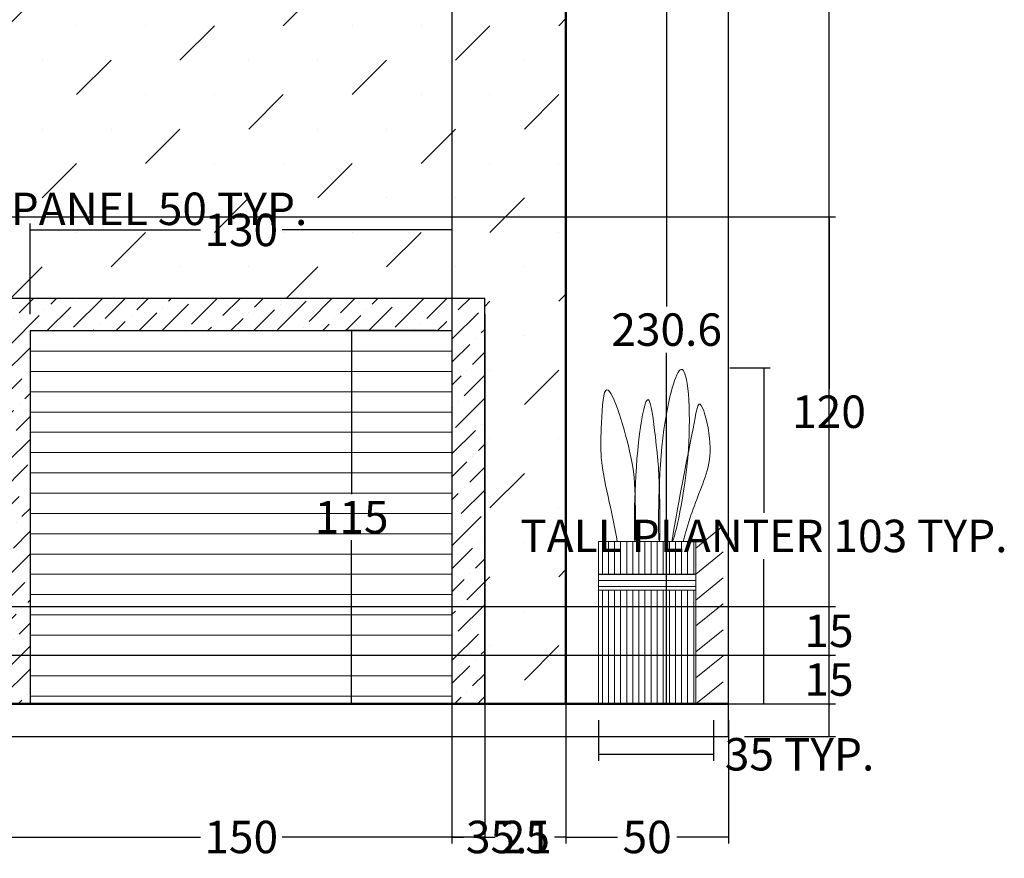
# Model space of a CAD drawing. Units: millimetres. Extents: x 301 to 1039, y -12 to 673.
# Tile 5 of 6: x 736 to 1039, y -12 to 246. Entities that reach past the tile are written whole.
import ezdxf

# ---------------------------------------------------------------- set-up
doc = ezdxf.new("R2010")
doc.units = ezdxf.units.MM
doc.header["$MEASUREMENT"] = 0
for name, color, linetype, lineweight in [('A-ANNO-DIMS', 2, 'Continuous', 18), ('A-DOOR', 4, 'Continuous', 25), ('A-DOOR-PATT', 8, 'Continuous', 13), ('A-ELEV', 8, 'Continuous', 25), ('A-WALL', 7, 'Continuous', 50), ('A-WALL-PATT', 9, 'Continuous', 13), ('L-PLNT', 3, 'Continuous', 18)]:
    doc.layers.add(name, color=color, linetype=linetype, lineweight=lineweight)
doc.styles.get("Standard").update_dxf_attribs({"font": 'arial.ttf'})
doc.dimstyles.get("Standard").update_dxf_attribs({"dimtxt": 10, "dimasz": 0.18, "dimexe": 2, "dimexo": 5, "dimgap": 2, "dimtad": 0, "dimtih": 1, "dimtoh": 1, "dimdec": 0, "dimzin": 0, "dimdsep": 46, "dimtxsty": 'Standard', "dimcen": 0.09, "dimadec": 0, "dimazin": 0, "dimtfac": 1, "dimtdec": 0, "dimtofl": 0, "dimtmove": 0, "dimatfit": 3, "dimfxl": 1, "dimtolj": 1, "dimtzin": 0, "dimarcsym": 0})

# ---------------------------------------------------------------- blocks, each defined once
blk = doc.blocks.new('*U1')
blk.add_line((0, 0), (6.81, -8.44))
blk = doc.blocks.new('*U2')
at = {"layer": 'L-PLNT', "color": 0, "linetype": 'ByBlock', "lineweight": -2, "transparency": 16777216, "rotation": 90}
for p in [(943.79, 83.09), (943.79, 75.09), (943.79, 67.09), (943.79, 59.09), (943.79, 51.09), (943.79, 43.09), (943.79, 35.09)]:
    blk.add_blockref('*U1', p, dxfattribs=at)
blk = doc.blocks.new('PLANTER-TALL')
for p, q in [((913.79, 35.09), (913.79, 85.09)), ((913.79, 85.09), (943.79, 85.09)), ((943.79, 85.09), (943.79, 35.09)), ((913.79, 75.09), (943.79, 75.09)), ((913.79, 70.09), (943.79, 70.09))]:
    blk.add_line(p, q)
for points, knots in [([(932.44, 85.09), (932.19, 88.91), (932, 117.56), (940.64, 148.58), (943.41, 110.75), (932.62, 67.84), (940.69, 108.37), (944.93, 130.41), (949.97, 112.97), (945.67, 102.5), (941.16, 90.48), (939.89, 85.09)], [190.612749, 190.612749, 190.612749, 190.612749, 217.894774, 237.177461, 261.995493, 290.738764, 329.494028, 333.833671, 341.635675, 361.055373, 377.63197, 377.63197, 377.63197, 377.63197]), ([(919.6, 85.09), (918.81, 89.12), (917.13, 97.69), (914.28, 109.64), (914.65, 119.96), (915.42, 140.89), (924.57, 111.13), (925.2, 100.17), (925.2, 87.12), (925.13, 85.09)], [0, 0, 0, 0, 12.444322, 26.420596, 35.223716, 47.132736, 67.219262, 83.208341, 95.201321, 95.201321, 95.201321, 95.201321]), ([(924.96, 85.09), (924.77, 89.03), (924.72, 111.77), (929.35, 134.6), (931.92, 112.35), (932.77, 102.84), (932.74, 87.27), (932.64, 85.09)], [102.717678, 102.717678, 102.717678, 102.717678, 128.408935, 139.329582, 151.017137, 169.163832, 183.363914, 183.363914, 183.363914, 183.363914])]:
    blk.add_open_spline(points, degree=3, knots=knots)
blk = doc.blocks.new('*D10')
at = {"layer": 'A-ANNO-DIMS', "color": 0, "lineweight": -2, "transparency": 16777216}
for p, q in [((633.79, 185.09), (633.79, 189.59)), ((683.79, 185.09), (683.79, 189.59)), ((633.97, 187.59), (683.61, 187.59)), ((683.79, 187.59), (683.97, 187.59))]:
    blk.add_line(p, q, dxfattribs=at)
at = {"layer": 'A-ANNO-DIMS', "color": 0, "transparency": 16777216}
for points in [[(633.97, 187.62), (633.97, 187.56), (633.79, 187.59)], [(683.61, 187.62), (683.61, 187.56), (683.79, 187.59)]]:
    blk.add_solid(points, dxfattribs=at)
at = {"layer": 'Defpoints', "color": 0, "transparency": 16777216}
for p in [(683.79, 187.59), (633.79, 180.09), (683.79, 180.09)]:
    blk.add_point(p, dxfattribs=at)
at = {"layer": 'A-ANNO-DIMS', "color": 0, "transparency": 16777216, "insert": (757.8, 187.59), "char_height": 10, "attachment_point": 5}
blk.add_mtext('\\A1;DOOR PANEL 50 TYP.', dxfattribs=at)
blk = doc.blocks.new('*D18')
at = {"layer": 'A-ANNO-DIMS', "color": 0, "lineweight": -2, "transparency": 16777216}
for p, q in [((954.2, 138.57), (966.72, 138.57)), ((964.72, 138.39), (964.72, 93.94)), ((964.72, 35.27), (964.72, 79.72)), ((954.2, 35.09), (966.72, 35.09))]:
    blk.add_line(p, q, dxfattribs=at)
at = {"layer": 'A-ANNO-DIMS', "color": 0, "transparency": 16777216}
for points in [[(964.69, 138.39), (964.75, 138.39), (964.72, 138.57)], [(964.69, 35.27), (964.75, 35.27), (964.72, 35.09)]]:
    blk.add_solid(points, dxfattribs=at)
at = {"layer": 'Defpoints', "color": 0, "transparency": 16777216}
for p in [(949.2, 138.57), (964.72, 138.57), (949.2, 35.09)]:
    blk.add_point(p, dxfattribs=at)
at = {"layer": 'A-ANNO-DIMS', "color": 0, "transparency": 16777216, "insert": (964.72, 86.83), "char_height": 10, "attachment_point": 5}
blk.add_mtext('\\A1;TALL PLANTER 103 TYP.', dxfattribs=at)
blk = doc.blocks.new('*D19')
at = {"layer": 'A-ANNO-DIMS', "color": 0, "lineweight": -2, "transparency": 16777216}
for p, q in [((913.79, 30.09), (913.79, 17.57)), ((949.2, 30.09), (949.2, 17.57)), ((913.97, 19.57), (949.02, 19.57)), ((949.2, 19.57), (949.38, 19.57))]:
    blk.add_line(p, q, dxfattribs=at)
at = {"layer": 'A-ANNO-DIMS', "color": 0, "transparency": 16777216}
for points in [[(913.97, 19.6), (913.97, 19.54), (913.79, 19.57)], [(949.02, 19.6), (949.02, 19.54), (949.2, 19.57)]]:
    blk.add_solid(points, dxfattribs=at)
at = {"layer": 'Defpoints', "color": 0, "transparency": 16777216}
for p in [(913.79, 35.09), (949.2, 35.09), (949.2, 19.57)]:
    blk.add_point(p, dxfattribs=at)
at = {"layer": 'A-ANNO-DIMS', "color": 0, "transparency": 16777216, "insert": (975.72, 19.57), "char_height": 10, "attachment_point": 5}
blk.add_mtext('\\A1;35 TYP.', dxfattribs=at)
blk = doc.blocks.new('*D20')
at = {"layer": 'A-ANNO-DIMS', "color": 0, "lineweight": -2, "transparency": 16777216}
for p, q in [((343.79, 30.09), (343.79, 668.09)), ((953.79, 30.09), (953.79, 668.09)), ((343.97, 666.09), (635.73, 666.09)), ((953.61, 666.09), (661.85, 666.09))]:
    blk.add_line(p, q, dxfattribs=at)
at = {"layer": 'A-ANNO-DIMS', "color": 0, "transparency": 16777216}
for points in [[(343.97, 666.12), (343.97, 666.06), (343.79, 666.09)], [(953.61, 666.12), (953.61, 666.06), (953.79, 666.09)]]:
    blk.add_solid(points, dxfattribs=at)
at = {"layer": 'Defpoints', "color": 0, "transparency": 16777216}
for p in [(953.79, 666.09), (343.79, 25.09), (953.79, 25.09)]:
    blk.add_point(p, dxfattribs=at)
at = {"layer": 'A-ANNO-DIMS', "color": 0, "transparency": 16777216, "insert": (648.79, 666.09), "char_height": 10, "attachment_point": 5}
blk.add_mtext('\\A1;610', dxfattribs=at)
blk = doc.blocks.new('*D21')
at = {"layer": 'A-ANNO-DIMS', "color": 0, "lineweight": -2, "transparency": 16777216}
for p, q in [((905.87, 635.09), (986.79, 635.09)), ((984.79, 634.91), (984.79, 337.19)), ((984.79, 25.27), (984.79, 322.98)), ((958.79, 25.09), (986.79, 25.09))]:
    blk.add_line(p, q, dxfattribs=at)
at = {"layer": 'A-ANNO-DIMS', "color": 0, "transparency": 16777216}
for points in [[(984.76, 634.91), (984.82, 634.91), (984.79, 635.09)], [(984.76, 25.27), (984.82, 25.27), (984.79, 25.09)]]:
    blk.add_solid(points, dxfattribs=at)
at = {"layer": 'Defpoints', "color": 0, "transparency": 16777216}
for p in [(900.87, 635.09), (984.79, 635.09), (953.79, 25.09)]:
    blk.add_point(p, dxfattribs=at)
at = {"layer": 'A-ANNO-DIMS', "color": 0, "transparency": 16777216, "insert": (984.79, 330.09), "char_height": 10, "attachment_point": 5}
blk.add_mtext('\\A1;610', dxfattribs=at)
blk = doc.blocks.new('*D28')
at = {"layer": 'A-ANNO-DIMS', "color": 0, "lineweight": -2, "transparency": 16777216}
for p, q in [((728.79, 155.09), (728.79, -7.91)), ((878.79, 155.09), (878.79, -7.91)), ((728.97, -5.91), (791.23, -5.91)), ((878.61, -5.91), (816.35, -5.91))]:
    blk.add_line(p, q, dxfattribs=at)
at = {"layer": 'A-ANNO-DIMS', "color": 0, "transparency": 16777216}
for points in [[(728.97, -5.88), (728.97, -5.94), (728.79, -5.91)], [(878.61, -5.88), (878.61, -5.94), (878.79, -5.91)]]:
    blk.add_solid(points, dxfattribs=at)
at = {"layer": 'Defpoints', "color": 0, "transparency": 16777216}
for p in [(728.79, 160.09), (878.79, 160.09), (878.79, -5.91)]:
    blk.add_point(p, dxfattribs=at)
at = {"layer": 'A-ANNO-DIMS', "color": 0, "transparency": 16777216, "insert": (803.79, -5.91), "char_height": 10, "attachment_point": 5}
blk.add_mtext('\\A1;150', dxfattribs=at)
blk = doc.blocks.new('*D29')
at = {"layer": 'A-ANNO-DIMS', "color": 0, "lineweight": -2, "transparency": 16777216}
for p, q in [((878.79, 30.09), (878.79, -7.91)), ((903.79, 30.09), (903.79, -7.91)), ((878.97, -5.91), (882, -5.91)), ((903.61, -5.91), (900.57, -5.91))]:
    blk.add_line(p, q, dxfattribs=at)
at = {"layer": 'A-ANNO-DIMS', "color": 0, "transparency": 16777216}
for points in [[(878.97, -5.88), (878.97, -5.94), (878.79, -5.91)], [(903.61, -5.88), (903.61, -5.94), (903.79, -5.91)]]:
    blk.add_solid(points, dxfattribs=at)
at = {"layer": 'Defpoints', "color": 0, "transparency": 16777216}
for p in [(878.79, 35.09), (903.79, 35.09), (903.79, -5.91)]:
    blk.add_point(p, dxfattribs=at)
at = {"layer": 'A-ANNO-DIMS', "color": 0, "transparency": 16777216, "insert": (891.29, -5.91), "char_height": 10, "attachment_point": 5}
blk.add_mtext('\\A1;25', dxfattribs=at)
blk = doc.blocks.new('*D30')
at = {"layer": 'A-ANNO-DIMS', "color": 0, "lineweight": -2, "transparency": 16777216}
for p, q in [((903.79, 30.09), (903.79, -7.91)), ((953.79, 30.09), (953.79, -7.91)), ((903.97, -5.91), (919.64, -5.91)), ((953.61, -5.91), (937.93, -5.91))]:
    blk.add_line(p, q, dxfattribs=at)
at = {"layer": 'A-ANNO-DIMS', "color": 0, "transparency": 16777216}
for points in [[(903.97, -5.88), (903.97, -5.94), (903.79, -5.91)], [(953.61, -5.88), (953.61, -5.94), (953.79, -5.91)]]:
    blk.add_solid(points, dxfattribs=at)
at = {"layer": 'Defpoints', "color": 0, "transparency": 16777216}
for p in [(903.79, 35.09), (953.79, 35.09), (953.79, -5.91)]:
    blk.add_point(p, dxfattribs=at)
at = {"layer": 'A-ANNO-DIMS', "color": 0, "transparency": 16777216, "insert": (928.79, -5.91), "char_height": 10, "attachment_point": 5}
blk.add_mtext('\\A1;50', dxfattribs=at)
blk = doc.blocks.new('*D38')
at = {"layer": 'A-ANNO-DIMS', "color": 0, "lineweight": -2, "transparency": 16777216}
for p, q in [((908.79, 265.67), (936.79, 265.67)), ((934.79, 265.49), (934.79, 157.49)), ((934.79, 35.27), (934.79, 143.27)), ((908.79, 35.09), (936.79, 35.09))]:
    blk.add_line(p, q, dxfattribs=at)
at = {"layer": 'A-ANNO-DIMS', "color": 0, "transparency": 16777216}
for points in [[(934.76, 265.49), (934.82, 265.49), (934.79, 265.67)], [(934.76, 35.27), (934.82, 35.27), (934.79, 35.09)]]:
    blk.add_solid(points, dxfattribs=at)
at = {"layer": 'Defpoints', "color": 0, "transparency": 16777216}
for p in [(903.79, 265.67), (903.79, 35.09), (934.79, 35.09)]:
    blk.add_point(p, dxfattribs=at)
at = {"layer": 'A-ANNO-DIMS', "color": 0, "transparency": 16777216, "insert": (934.79, 150.38), "char_height": 10, "attachment_point": 5}
blk.add_mtext('\\A1;230.6', dxfattribs=at)
blk = doc.blocks.new('*D41')
at = {"layer": 'A-ANNO-DIMS', "color": 0, "lineweight": -2, "transparency": 16777216}
for p, q in [((863.79, 150.09), (835.79, 150.09)), ((837.79, 149.91), (837.79, 99.69)), ((837.79, 35.27), (837.79, 85.48)), ((863.79, 35.09), (835.79, 35.09))]:
    blk.add_line(p, q, dxfattribs=at)
at = {"layer": 'A-ANNO-DIMS', "color": 0, "transparency": 16777216}
for points in [[(837.76, 149.91), (837.82, 149.91), (837.79, 150.09)], [(837.76, 35.27), (837.82, 35.27), (837.79, 35.09)]]:
    blk.add_solid(points, dxfattribs=at)
at = {"layer": 'Defpoints', "color": 0, "transparency": 16777216}
for p in [(837.79, 150.09), (868.79, 150.09), (868.79, 35.09)]:
    blk.add_point(p, dxfattribs=at)
at = {"layer": 'A-ANNO-DIMS', "color": 0, "transparency": 16777216, "insert": (837.79, 92.59), "char_height": 10, "attachment_point": 5}
blk.add_mtext('\\A1;115', dxfattribs=at)
blk = doc.blocks.new('*D42')
at = {"layer": 'A-ANNO-DIMS', "color": 0, "lineweight": -2, "transparency": 16777216}
for p, q in [((738.79, 155.09), (738.79, 183.09)), ((868.79, 155.09), (868.79, 183.09)), ((738.97, 181.09), (791.23, 181.09)), ((868.61, 181.09), (816.35, 181.09))]:
    blk.add_line(p, q, dxfattribs=at)
at = {"layer": 'A-ANNO-DIMS', "color": 0, "transparency": 16777216}
for points in [[(738.97, 181.12), (738.97, 181.06), (738.79, 181.09)], [(868.61, 181.12), (868.61, 181.06), (868.79, 181.09)]]:
    blk.add_solid(points, dxfattribs=at)
at = {"layer": 'Defpoints', "color": 0, "transparency": 16777216}
for p in [(868.79, 181.09), (738.79, 150.09), (868.79, 150.09)]:
    blk.add_point(p, dxfattribs=at)
at = {"layer": 'A-ANNO-DIMS', "color": 0, "transparency": 16777216, "insert": (803.79, 181.09), "char_height": 10, "attachment_point": 5}
blk.add_mtext('\\A1;130', dxfattribs=at)
blk = doc.blocks.new('*D69')
at = {"layer": 'A-ANNO-DIMS', "color": 0, "lineweight": -2, "transparency": 16777216}
for p, q in [((708.788413, 50.088152), (986.788413, 50.088152)), ((984.788413, 50.268152), (984.788413, 50.448152)), ((708.788413, 35.088152), (986.788413, 35.088152)), ((984.788413, 34.908152), (984.788413, 34.728152))]:
    blk.add_line(p, q, dxfattribs=at)
at = {"layer": 'A-ANNO-DIMS', "color": 0, "transparency": 16777216}
for points in [[(984.758413, 50.268152), (984.818413, 50.268152), (984.788413, 50.088152)], [(984.758413, 34.908152), (984.818413, 34.908152), (984.788413, 35.088152)]]:
    blk.add_solid(points, dxfattribs=at)
at = {"layer": 'Defpoints', "color": 0, "transparency": 16777216}
for p in [(703.788413, 50.088152), (984.788413, 50.088152), (703.788413, 35.088152)]:
    blk.add_point(p, dxfattribs=at)
at = {"layer": 'A-ANNO-DIMS', "color": 0, "transparency": 16777216, "insert": (984.788413, 42.588152), "char_height": 10, "attachment_point": 5}
blk.add_mtext('\\A1;15', dxfattribs=at)
blk = doc.blocks.new('*D70')
at = {"layer": 'A-ANNO-DIMS', "color": 0, "lineweight": -2, "transparency": 16777216}
for p, q in [((708.788413, 65.088152), (986.788413, 65.088152)), ((984.788413, 65.268152), (984.788413, 65.448152)), ((708.788413, 50.088152), (986.788413, 50.088152)), ((984.788413, 49.908152), (984.788413, 49.728152))]:
    blk.add_line(p, q, dxfattribs=at)
at = {"layer": 'A-ANNO-DIMS', "color": 0, "transparency": 16777216}
for points in [[(984.758413, 65.268152), (984.818413, 65.268152), (984.788413, 65.088152)], [(984.758413, 49.908152), (984.818413, 49.908152), (984.788413, 50.088152)]]:
    blk.add_solid(points, dxfattribs=at)
at = {"layer": 'Defpoints', "color": 0, "transparency": 16777216}
for p in [(703.788413, 65.088152), (984.788413, 65.088152), (703.788413, 50.088152)]:
    blk.add_point(p, dxfattribs=at)
at = {"layer": 'A-ANNO-DIMS', "color": 0, "transparency": 16777216, "insert": (984.788413, 57.588152), "char_height": 10, "attachment_point": 5}
blk.add_mtext('\\A1;15', dxfattribs=at)
blk = doc.blocks.new('*D71')
at = {"layer": 'A-ANNO-DIMS', "color": 0, "lineweight": -2, "transparency": 16777216}
for p, q in [((693.79, 185.09), (986.79, 185.09)), ((984.79, 184.91), (984.79, 132.19)), ((984.79, 65.27), (984.79, 117.98)), ((693.79, 65.09), (986.79, 65.09))]:
    blk.add_line(p, q, dxfattribs=at)
at = {"layer": 'A-ANNO-DIMS', "color": 0, "transparency": 16777216}
for points in [[(984.76, 184.91), (984.82, 184.91), (984.79, 185.09)], [(984.76, 65.27), (984.82, 65.27), (984.79, 65.09)]]:
    blk.add_solid(points, dxfattribs=at)
at = {"layer": 'Defpoints', "color": 0, "transparency": 16777216}
for p in [(688.79, 185.09), (984.79, 185.09), (688.79, 65.09)]:
    blk.add_point(p, dxfattribs=at)
at = {"layer": 'A-ANNO-DIMS', "color": 0, "transparency": 16777216, "insert": (984.79, 125.09), "char_height": 10, "attachment_point": 5}
blk.add_mtext('\\A1;120', dxfattribs=at)
blk = doc.blocks.new('*D75')
at = {"layer": 'A-ANNO-DIMS', "color": 0, "lineweight": -2, "transparency": 16777216}
for p, q in [((868.69, 285.26), (868.69, -7.91)), ((903.79, 260.67), (903.79, -7.91)), ((868.87, -5.91), (872.22, -5.91)), ((903.61, -5.91), (900.26, -5.91))]:
    blk.add_line(p, q, dxfattribs=at)
at = {"layer": 'A-ANNO-DIMS', "color": 0, "transparency": 16777216}
for points in [[(868.87, -5.88), (868.87, -5.94), (868.69, -5.91)], [(903.61, -5.88), (903.61, -5.94), (903.79, -5.91)]]:
    blk.add_solid(points, dxfattribs=at)
at = {"layer": 'Defpoints', "color": 0, "transparency": 16777216}
for p in [(868.69, 290.26), (903.79, 265.67), (903.79, -5.91)]:
    blk.add_point(p, dxfattribs=at)
at = {"layer": 'A-ANNO-DIMS', "color": 0, "transparency": 16777216, "insert": (886.24, -5.91), "char_height": 10, "attachment_point": 5}
blk.add_mtext('\\A1;35.1', dxfattribs=at)

msp = doc.modelspace()

# ---------------------------------------------------------------- hatches: boundary and pattern name
at = {"layer": 'A-DOOR-PATT'}
h = msp.add_hatch(dxfattribs=at)
h.set_pattern_fill('ANSI31', color=256, scale=50, angle=135)
h.paths.add_polyline_path([(868.788, 150.088), (738.788, 150.088), (738.788, 35.088), (868.788, 35.088)])
at = {"layer": 'A-WALL-PATT'}
h = msp.add_hatch(dxfattribs=at)
h.set_pattern_fill('MUDST', color=256, scale=60, angle=45)
edge = h.paths.add_edge_path()
edge.add_line((703.788, 505.088), (403.788, 505.088))
edge.add_line((403.788, 505.088), (403.788, 335.088))
edge.add_line((403.788, 335.088), (448.788, 335.088))
edge.add_line((448.788, 335.088), (448.788, 400.52))
edge.add_line((448.788, 400.52), (448.788, 440.088))
edge.add_line((448.788, 440.088), (633.788, 440.088))
edge.add_line((633.788, 440.088), (633.788, 400.52))
edge.add_line((633.788, 400.52), (633.788, 335.088))
edge.add_line((633.788, 335.088), (673.88, 335.088))
edge.add_spline(control_points=[(673.88, 335.088), (673.929, 335.734), (674.283, 339.462), (675.587, 346.794), (678.602, 339.909), (679.226, 336.718), (679.369, 335.088)], knot_values=[26.7052686, 26.7052686, 26.7052686, 26.7052686, 28.3156814, 35.5227919, 39.6456178, 44.5318346, 44.5318346, 44.5318346, 44.5318346], degree=3, periodic=0)
edge.add_line((679.369, 335.088), (703.788, 335.088))
edge.add_line((703.788, 335.088), (703.788, 505.088))
h.paths.add_polyline_path([(681.292, 397.334, -1), (651.292, 397.334, -1)], flags=16)
h.paths.add_polyline_path([(679.292, 397.334, -1), (653.292, 397.334, -1)], flags=0)
h.paths.add_polyline_path([(448.788, 333.088), (403.788, 333.088), (403.788, 285.088), (448.788, 285.088)])
h.paths.add_polyline_path([(613.788, 260.088), (713.788, 260.088), (713.788, 285.088), (403.788, 285.088), (393.788, 285.088), (393.788, 35.088), (403.788, 35.088), (613.788, 35.088)])
h.paths.add_polyline_path([(578.788, 215.088), (578.788, 105.088), (428.788, 105.088), (428.788, 215.088)], flags=16)
h.paths.add_polyline_path([(501.288, 210.088), (501.288, 185.088), (433.788, 185.088), (433.788, 210.088)], flags=0)
h.paths.add_polyline_path([(501.288, 180.088), (501.288, 110.088), (433.788, 110.088), (433.788, 180.088)], flags=0)
h.paths.add_polyline_path([(506.288, 210.088), (573.788, 210.088), (573.788, 185.088), (506.288, 185.088)], flags=0)
h.paths.add_polyline_path([(506.288, 180.088), (573.788, 180.088), (573.788, 110.088), (506.288, 110.088)], flags=0)
edge = h.paths.add_edge_path()
edge.add_spline(control_points=[(675.148, 309.006), (675.282, 309.92), (671.965, 311.304), (670.019, 313.17), (668.379, 316.485), (667.076, 320.028), (669.149, 324.142), (672.687, 322.877), (673.644, 321.553), (673.786, 321.296)], knot_values=[12.4980994, 12.4980994, 12.4980994, 12.4980994, 15.7345293, 18.1242776, 22.0598536, 26.1694355, 29.2709867, 33.3603853, 34.273637, 34.273637, 34.273637, 34.273637], degree=3, periodic=0)
edge.add_spline(control_points=[(673.786, 321.296), (673.373, 322.666), (672.565, 324.662), (673.805, 325.84), (674.246, 326.099)], knot_values=[12.3304253, 12.3304253, 12.3304253, 12.3304253, 16.1943692, 17.6683934, 17.6683934, 17.6683934, 17.6683934], degree=3, periodic=0)
edge.add_spline(control_points=[(674.246, 326.099), (673.92, 328.298), (673.697, 330.39), (673.774, 333.088)], knot_values=[46.2924512, 46.2924512, 46.2924512, 46.2924512, 53.8278009, 53.8278009, 53.8278009, 53.8278009], degree=3, periodic=0)
edge.add_line((673.774, 333.088), (648.788, 333.088))
edge.add_line((648.788, 333.088), (648.788, 285.088))
edge.add_line((648.788, 285.088), (666.788, 285.088))
edge.add_line((666.788, 285.088), (664.215, 309.96))
edge.add_arc((676.288, 385.148), 76.15, 260.87778, 269.14183)
edge = h.paths.add_edge_path()
edge.add_line((703.788, 333.088), (679.453, 333.088))
edge.add_spline(control_points=[(679.453, 333.088), (679.452, 331.277), (679.21, 329.205), (678.936, 327.067), (678.889, 326.706)], knot_values=[17.8386285, 17.8386285, 17.8386285, 17.8386285, 23.5111371, 24.6594022, 24.6594022, 24.6594022, 24.6594022], degree=3, periodic=0)
edge.add_spline(control_points=[(678.889, 326.706), (678.729, 326.741), (678.565, 326.771), (678.396, 326.794)], knot_values=[21.2892091, 21.2892091, 21.2892091, 21.2892091, 21.7264211, 21.7264211, 21.7264211, 21.7264211], degree=3, periodic=0)
edge.add_spline(control_points=[(678.396, 326.794), (678.233, 326.816), (678.067, 326.832), (677.898, 326.842)], knot_values=[20.8675669, 20.8675669, 20.8675669, 20.8675669, 21.2892091, 21.2892091, 21.2892091, 21.2892091], degree=3, periodic=0)
edge.add_spline(control_points=[(677.898, 326.842), (676.995, 326.898), (676.024, 326.786), (675.195, 326.517)], knot_values=[18.611077, 18.611077, 18.611077, 18.611077, 20.8675669, 20.8675669, 20.8675669, 20.8675669], degree=3, periodic=0)
edge.add_spline(control_points=[(675.195, 326.517), (675.029, 326.464), (674.869, 326.404), (674.716, 326.337)], knot_values=[18.1593829, 18.1593829, 18.1593829, 18.1593829, 18.611077, 18.611077, 18.611077, 18.611077], degree=3, periodic=0)
edge.add_spline(control_points=[(674.716, 326.337), (674.55, 326.265), (674.392, 326.186), (674.246, 326.099)], knot_values=[17.6683934, 17.6683934, 17.6683934, 17.6683934, 18.1593829, 18.1593829, 18.1593829, 18.1593829], degree=3, periodic=0)
edge.add_spline(control_points=[(674.246, 326.099), (673.805, 325.84), (672.565, 324.662), (673.373, 322.666), (673.786, 321.296)], knot_values=[12.3304253, 12.3304253, 12.3304253, 12.3304253, 13.8044495, 17.6683934, 17.6683934, 17.6683934, 17.6683934], degree=3, periodic=0)
edge.add_spline(control_points=[(673.786, 321.296), (674.162, 320.613), (674.301, 319.823), (674.341, 318.987)], knot_values=[10.0649388, 10.0649388, 10.0649388, 10.0649388, 12.4980994, 12.4980994, 12.4980994, 12.4980994], degree=3, periodic=0)
edge.add_spline(control_points=[(674.341, 318.987), (674.206, 319.737), (674.024, 320.504), (673.786, 321.296)], knot_values=[10.094462, 10.094462, 10.094462, 10.094462, 12.3304253, 12.3304253, 12.3304253, 12.3304253], degree=3, periodic=0)
edge.add_spline(control_points=[(673.786, 321.296), (673.644, 321.553), (672.687, 322.877), (669.149, 324.142), (667.076, 320.028), (668.379, 316.485), (670.019, 313.17), (671.965, 311.304), (675.282, 309.92), (675.148, 309.006)], knot_values=[12.4980994, 12.4980994, 12.4980994, 12.4980994, 13.4113511, 17.5007497, 20.6023009, 24.7118828, 28.6474588, 31.0372071, 34.273637, 34.273637, 34.273637, 34.273637], degree=3, periodic=0)
edge.add_arc((676.288, 385.148), 76.15, 260.87778, 269.14183, ccw=False)
edge.add_line((664.215, 309.96), (666.788, 285.088))
edge.add_line((666.788, 285.088), (703.788, 285.088))
edge.add_line((703.788, 285.088), (703.788, 333.088))
h.paths.add_polyline_path([(687.234, 308.777), (684.887, 286.088), (667.69, 286.088), (665.343, 308.777, 0.0712952)], flags=16)
h.paths.add_polyline_path([(903.788, 265.672), (713.788, 265.672), (713.788, 260.088), (703.788, 260.088), (703.788, 35.088), (728.788, 35.088), (728.788, 160.088), (878.788, 160.088), (878.788, 35.088), (903.788, 35.088)])
h = msp.add_hatch(dxfattribs=at)
h.set_pattern_fill('ANSI36', color=256, scale=40)
h.paths.add_polyline_path([(878.788, 160.088), (728.788, 160.088), (728.788, 35.088), (738.788, 35.088), (738.788, 150.088), (868.788, 150.088), (868.788, 35.088), (878.788, 35.088)])
at = {"layer": 'L-PLNT'}
h = msp.add_hatch(dxfattribs=at)
h.set_pattern_fill('ANSI31', color=256, scale=15, angle=45)
edge = h.paths.add_edge_path()
edge.add_line((943.788, 85.088), (936.592, 85.088))
edge.add_spline(control_points=[(936.592, 85.088), (936.558, 85.041), (936.535, 85.042), (936.521, 85.088)], knot_values=[290.7387637, 290.7387637, 290.7387637, 290.7387637, 292.5163462, 292.5163462, 292.5163462, 292.5163462], degree=3, periodic=0)
edge.add_line((936.521, 85.088), (913.788, 85.088))
edge.add_line((913.788, 85.088), (913.788, 75.088))
edge.add_line((913.788, 75.088), (943.788, 75.088))
edge.add_line((943.788, 75.088), (943.788, 85.088))
h.paths.add_polyline_path([(943.788, 70.088), (913.788, 70.088), (913.788, 35.088), (943.788, 35.088)])
h = msp.add_hatch(dxfattribs=at)
h.set_pattern_fill('ANSI31', color=256, scale=15, angle=135)
h.paths.add_polyline_path([(943.788, 75.088), (913.788, 75.088), (913.788, 70.088), (943.788, 70.088)])

# ---------------------------------------------------------------- linework, layer by layer
at = {"layer": 'A-DOOR'}
for p, q in [((728.788, 160.088), (878.788, 160.088)), ((878.788, 35.088), (878.788, 160.088)), ((738.788, 150.088), (868.788, 150.088)), ((738.788, 150.088), (738.788, 35.088)), ((868.788, 35.088), (868.788, 150.088))]:
    msp.add_line(p, q, dxfattribs=at)
at = {"layer": 'A-ELEV'}
for p, q in [((953.788, 25.088), (953.788, 35.088)), ((618.788, 25.088), (953.788, 25.088))]:
    msp.add_line(p, q, dxfattribs=at)
at = {"layer": 'A-WALL'}
for p, q in [((903.788, 35.088), (903.788, 585.088)), ((953.788, 35.088), (403.788, 35.088)), ((953.788, 35.088), (903.788, 35.088))]:
    msp.add_line(p, q, dxfattribs=at)

# ---------------------------------------------------------------- block references
at = {"layer": 'L-PLNT'}
for name in ['PLANTER-TALL', '*U2']:
    msp.add_blockref(name, (0, 0), dxfattribs=at)

# ---------------------------------------------------------------- dimensions: what is measured, and where the dimension line sits
at = {"layer": 'A-ANNO-DIMS'}
for base, p1, p2, override, picture, middle in [((953.788, 666.088), (343.788, 25.088), (953.788, 25.088), {"dimdec": 0, "dimlfac": 1, "dimrnd": 0, "dimzin": 0, "dimdsep": 46, "dimlunit": 2}, '*D20', (648.788, 666.088)), ((903.788, -5.912), (868.687, 290.264), (903.788, 265.672), {"dimdec": 1, "dimlfac": 1, "dimrnd": 0, "dimzin": 0, "dimdsep": 46, "dimlunit": 2}, '*D75', (886.238, -5.912)), ((868.788, 181.088), (738.788, 150.088), (868.788, 150.088), {"dimdec": 0, "dimlfac": 1, "dimrnd": 0, "dimzin": 0, "dimdsep": 46, "dimlunit": 2}, '*D42', (803.788, 181.088)), ((878.788, -5.912), (728.788, 160.088), (878.788, 160.088), {"dimdec": 0, "dimlfac": 1, "dimrnd": 0, "dimzin": 0, "dimdsep": 46, "dimlunit": 2}, '*D28', (803.788, -5.912)), ((903.788, -5.912), (878.788, 35.088), (903.788, 35.088), {"dimdec": 0, "dimlfac": 1, "dimrnd": 0, "dimzin": 0, "dimdsep": 46, "dimlunit": 2}, '*D29', (891.288, -5.912)), ((953.788, -5.912), (903.788, 35.088), (953.788, 35.088), {"dimdec": 0, "dimlfac": 1, "dimrnd": 0, "dimzin": 0, "dimdsep": 46, "dimlunit": 2}, '*D30', (928.788, -5.912))]:
    dim = msp.add_linear_dim(base=base, p1=p1, p2=p2, dimstyle='Standard', override=override, dxfattribs=at)
    dim.commit()
    dim.dimension.update_dxf_attribs({"geometry": picture, "text_midpoint": middle})
for base, p1, p2, angle, override, picture, middle in [((984.788, 635.088), (953.788, 25.088), (900.87, 635.088), 90, {"dimdec": 0, "dimlfac": 1, "dimrnd": 0, "dimzin": 0, "dimdsep": 46, "dimlunit": 2}, '*D21', (984.788, 330.088)), ((934.788, 35.088), (903.788, 265.672), (903.788, 35.088), 270, {"dimdec": 1, "dimlfac": 1, "dimrnd": 0, "dimzin": 0, "dimdsep": 46, "dimlunit": 2}, '*D38', (934.788, 150.38)), ((984.788, 185.088), (688.788, 65.088), (688.788, 185.088), 90, {"dimdec": 0, "dimlfac": 1, "dimrnd": 0, "dimzin": 0, "dimdsep": 46, "dimlunit": 2}, '*D71', (984.788, 125.088)), ((837.788, 150.088), (868.788, 35.088), (868.788, 150.088), 90, {"dimdec": 0, "dimlfac": 1, "dimrnd": 0, "dimzin": 0, "dimdsep": 46, "dimlunit": 2}, '*D41', (837.788, 92.588)), ((984.788, 65.088), (703.788, 50.088), (703.788, 65.088), 90, {"dimdec": 0, "dimlfac": 1, "dimrnd": 0, "dimzin": 0, "dimdsep": 46, "dimlunit": 2}, '*D70', (984.788, 57.588)), ((984.788, 50.088), (703.788, 35.088), (703.788, 50.088), 90, {"dimdec": 0, "dimlfac": 1, "dimrnd": 0, "dimzin": 0, "dimdsep": 46, "dimlunit": 2}, '*D69', (984.788, 42.588))]:
    dim = msp.add_linear_dim(base=base, p1=p1, p2=p2, angle=angle, dimstyle='Standard', override=override, dxfattribs=at)
    dim.commit()
    dim.dimension.update_dxf_attribs({"geometry": picture, "text_midpoint": middle})
for base, p1, p2, text, picture, middle in [((683.788, 187.588), (633.788, 180.088), (683.788, 180.088), 'DOOR PANEL <> TYP.', '*D10', (757.8, 187.588)), ((949.203, 19.566), (913.788, 35.088), (949.203, 35.088), '<> TYP.', '*D19', (975.718, 19.566))]:
    dim = msp.add_linear_dim(base=base, p1=p1, p2=p2, text=text, dimstyle='Standard', override={"dimdec": 0, "dimrnd": 0, "dimzin": 0, "dimlunit": 2}, dxfattribs=at)
    dim.commit()
    dim.dimension.update_dxf_attribs({"geometry": picture, "text_midpoint": middle})
dim = msp.add_linear_dim(base=(964.725, 138.566), p1=(949.203, 35.088), p2=(949.203, 138.566), angle=90, text='TALL PLANTER <> TYP.', dimstyle='Standard', override={"dimdec": 0, "dimrnd": 0, "dimzin": 0, "dimlunit": 2}, dxfattribs=at)
dim.commit()
dim.dimension.update_dxf_attribs({"geometry": '*D18', "text_midpoint": (964.725, 86.827)})

doc.saveas('drawing.dxf')
